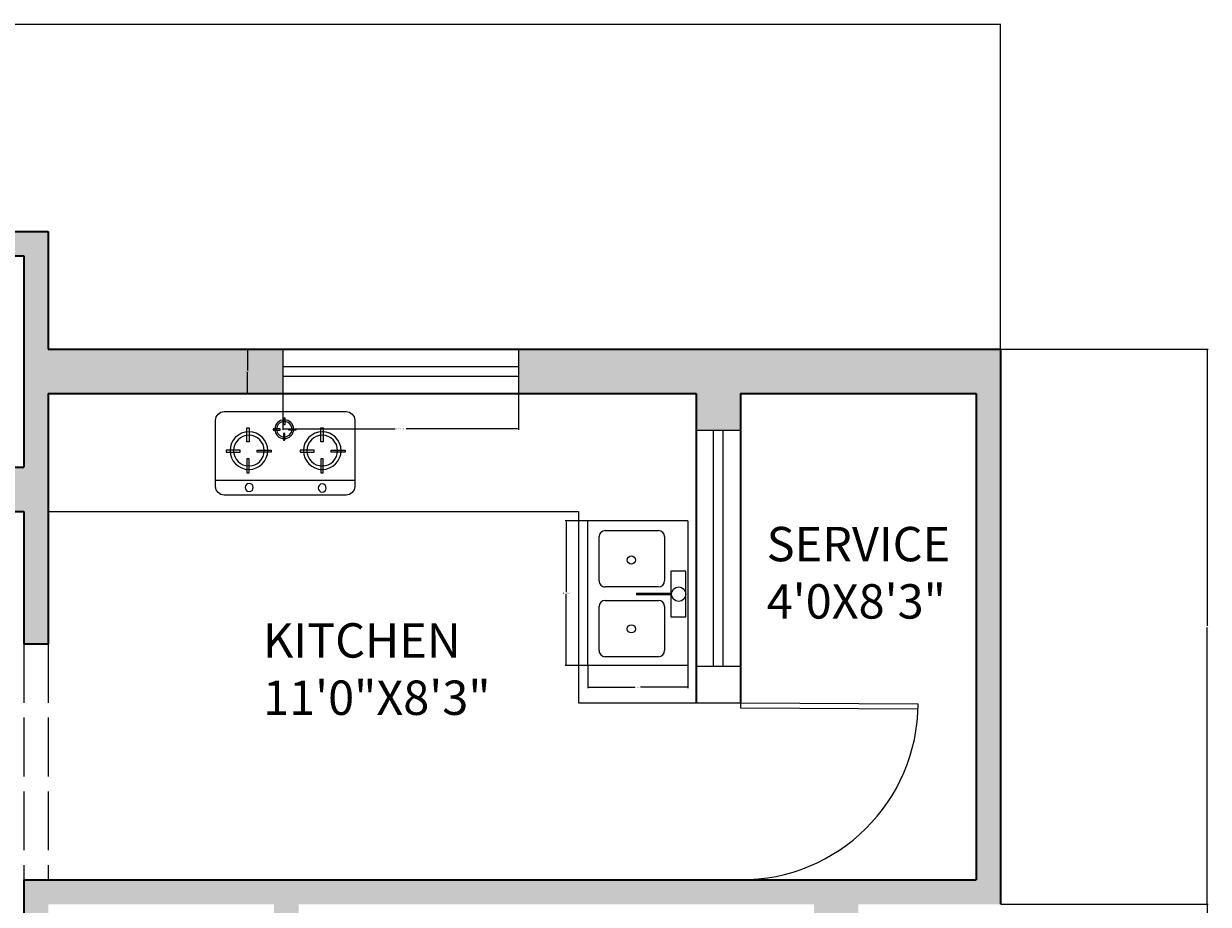
# Model space of a CAD drawing. Units: inches. Extents: x 2540 to 3167, y 3083 to 4007.
# Tile 15 of 15: x 2926 to 3167, y 3828 to 4007. Entities that reach past the tile are written whole.
import ezdxf

# ---------------------------------------------------------------- set-up
doc = ezdxf.new("R2010")
doc.units = ezdxf.units.IN
doc.linetypes.add('ACAD_ISO02W100', pattern=[15, 12, -3])
for name, color, linetype, lineweight in [('A-ANNO-DIMS', 2, 'Continuous', 18), ('A-AREA-IDEN', 7, 'Continuous', 18), ('A-DOOR', 4, 'Continuous', 18), ('A-EQPM', 9, 'Continuous', 18), ('A-FLOR-CASE', 9, 'Continuous', 18), ('A-FLOR-FIXT', 9, 'Continuous', 18), ('A-GLAZ', 4, 'Continuous', 18)]:
    doc.layers.add(name, color=color, linetype=linetype, lineweight=lineweight)
for name, color, linetype, lineweight, true_color in [('A-WALL', 143, 'Continuous', 35, 0x7aafdf), ('A-WALL-OVHD', 143, 'ACAD_ISO02W100', 18, 0x7aafdf), ('A-WALL-PATT', 143, 'Continuous', 13, 0x7aafdf)]:
    doc.layers.add(name, color=color, linetype=linetype, lineweight=lineweight, true_color=true_color)
doc.styles.get("Standard").update_dxf_attribs({"font": 'arial.ttf'})
doc.dimstyles.get("Standard").update_dxf_attribs({"dimtxt": 0.18, "dimasz": 0.18, "dimexe": 0.18, "dimexo": 0.0625, "dimgap": 0.09, "dimtad": 0, "dimtih": 1, "dimtoh": 1, "dimdec": 4, "dimzin": 0, "dimdsep": 46, "dimtxsty": 'Standard', "dimcen": 0.09, "dimadec": 0, "dimazin": 0, "dimtfac": 1, "dimtdec": 4, "dimtofl": 0, "dimtmove": 0, "dimatfit": 3, "dimfxl": 1, "dimtolj": 1, "dimtzin": 0, "dimarcsym": 0})

# ---------------------------------------------------------------- blocks, each defined once
blk = doc.blocks.new('A$C2A3C6842')
for p, q in [((45, 432), (675, 432)), ((0, 45), (0, 387)), ((351.6, 363.3), (351.6, 398.9)), ((351.6, 398.9), (357.3, 398.9)), ((357.3, 398.9), (357.3, 363.3)), ((720, 387), (720, 45)), ((161.8, 346.9), (173.2, 346.9)), ((161.8, 275.6), (161.8, 346.9)), ((173.2, 346.9), (173.2, 275.6)), ((298.4, 341.9), (298.4, 336.2)), ((334, 341.9), (298.4, 341.9)), ((298.4, 336.2), (334, 336.2)), ((334, 336.2), (334, 341.9)), ((357.3, 363.3), (351.6, 363.3)), ((357.3, 318.8), (351.6, 318.8)), ((351.6, 318.8), (351.6, 283.1)), ((357.3, 283.1), (357.3, 318.8)), ((378.5, 336.2), (378.5, 341.9)), ((378.5, 341.9), (414.2, 341.9)), ((414.2, 336.2), (378.5, 336.2)), ((414.2, 341.9), (414.2, 336.2)), ((544.7, 346.9), (556.1, 346.9)), ((544.7, 275.6), (544.7, 346.9)), ((556.1, 346.9), (556.1, 275.6)), ((173.2, 275.6), (161.8, 275.6)), ((351.6, 283.1), (357.3, 283.1)), ((556.1, 275.6), (544.7, 275.6)), ((55.3, 232.9), (55.3, 221.5)), ((126.6, 232.9), (55.3, 232.9)), ((55.3, 221.5), (126.6, 221.5)), ((126.6, 221.5), (126.6, 232.9)), ((173.2, 186.6), (161.8, 186.6)), ((161.8, 186.6), (161.8, 115.3)), ((173.2, 115.3), (173.2, 186.6)), ((215.6, 221.5), (215.6, 232.9)), ((215.6, 232.9), (286.9, 232.9)), ((286.9, 221.5), (215.6, 221.5)), ((286.9, 232.9), (286.9, 221.5)), ((438.2, 232.9), (438.2, 221.5)), ((509.5, 232.9), (438.2, 232.9)), ((438.2, 221.5), (509.5, 221.5)), ((509.5, 221.5), (509.5, 232.9)), ((556.1, 186.6), (544.7, 186.6)), ((544.7, 186.6), (544.7, 115.3)), ((556.1, 115.3), (556.1, 186.6)), ((598.5, 232.9), (669.8, 232.9)), ((598.5, 221.5), (598.5, 232.9)), ((669.8, 221.5), (598.5, 221.5)), ((669.8, 232.9), (669.8, 221.5)), ((1.2, 76.7), (719.9, 76.7)), ((161.8, 115.3), (173.2, 115.3)), ((544.7, 115.3), (556.1, 115.3)), ((675, 0), (45, 0))]:
    blk.add_line(p, q)
at = {"extrusion": (0, -1e-16, -1)}
for centre, major_axis, start_param, end_param in [((45, 387), (31.8, 31.8), 3.926991, 5.497787), ((172.2, 229.8), (-97.3, 0.1), -0.001099, 6.282086), ((551.8, 229.8), (-97.3, 0.1), -0.001099, 6.282086), ((173.7, 39), (-14.8, 14.8), 5.497787, 11.780972)]:
    blk.add_ellipse(centre, major_axis=major_axis, ratio=1, start_param=start_param, end_param=end_param, dxfattribs=at)
at = {"extrusion": (0, 1e-16, -1)}
blk.add_ellipse((675, 387), major_axis=(-31.8, 31.8), ratio=1, start_param=0.785398, end_param=2.356194, dxfattribs=at)
at = {"extrusion": (-1e-16, -1e-16, -1)}
blk.add_ellipse((355.1, 340.4), major_axis=(48.7, 0.1), ratio=1, start_param=3.144125, end_param=9.42731, dxfattribs=at)
at = {"extrusion": (-1e-16, 0, -1)}
for centre, major_axis, start_param, end_param in [((355.1, 340.4), (-39.7, 0), -0.000334, 6.282851), ((45, 45), (-31.8, 31.8), 3.926991, 5.497787)]:
    blk.add_ellipse(centre, major_axis=major_axis, ratio=1, start_param=start_param, end_param=end_param, dxfattribs=at)
at = {"extrusion": (-1e-16, -4e-16, -1)}
for centre in [(172.2, 229.8), (551.8, 229.8)]:
    blk.add_ellipse(centre, major_axis=(-79.3, 0), ratio=1, start_param=-0.0002116186602152, end_param=6.282973688519371, dxfattribs=at)
at = {"extrusion": (2e-16, -2e-16, -1)}
blk.add_ellipse((551.4, 36.4), major_axis=(14.8, 14.8), ratio=1, start_param=3.926991, end_param=10.210176, dxfattribs=at)
at = {"extrusion": (-2e-16, 1e-16, -1)}
blk.add_ellipse((675, 45), major_axis=(31.8, 31.8), ratio=1, start_param=0.785398, end_param=2.356194, dxfattribs=at)
at = {"text_generation_flag": 4, "flags": 9}
for tag in ['XSIZE', 'YSIZE']:
    blk.add_attdef(tag, (361.3, 264.9), '', height=0.45, rotation=180, dxfattribs=at)
blk = doc.blocks.new('A$C3AD04490')
for p, q in [((0, 640.7), (0, 0)), ((0, 640.7), (924.9, 640.7)), ((614, 627.3), (322.5, 627.3)), ((322.5, 627.3), (322.5, 531.5)), ((614, 531.5), (614, 627.3)), ((924.9, 640.7), (924.9, 0)), ((322.5, 531.5), (614, 531.5)), ((462.6, 311.9), (462.6, 537.2)), ((473.8, 536.8), (473.8, 311.9)), ((101.4, 490.5), (383.1, 490.5)), ((547.9, 490.5), (829.6, 490.5)), ((62.3, 110.9), (62.3, 451.4)), ((422.3, 451.4), (422.3, 110.9)), ((508.8, 110.9), (508.8, 451.4)), ((868.8, 451.4), (868.8, 110.9)), ((463.4, 310.9), (474.3, 310.9)), ((383.1, 71.7), (101.4, 71.7)), ((829.6, 71.7), (547.9, 71.7)), ((924.9, 0), (0, 0))]:
    blk.add_line(p, q)
for centre, radius in [((469, 581.2), 45.9), ((250.7, 278.1), 26.4), ((690.5, 278.1), 26.4)]:
    blk.add_circle(centre, radius)
for centre, start, end in [((101.4, 451.4), 90, 180), ((383.1, 451.4), 0, 90), ((547.9, 451.4), 90, 180), ((829.6, 451.4), 0, 90), ((101.4, 110.9), 180, 270), ((383.1, 110.9), 270, 0), ((547.9, 110.9), 180, 270), ((829.6, 110.9), 270, 0)]:
    blk.add_arc(centre, 39.1, start, end)
blk = doc.blocks.new('WIN-48IN')
for p, q in [((0, 48), (9, 48)), ((3.5, 0), (3.5, 48)), ((5.5, 0), (5.5, 48)), ((0, 0), (9, 0))]:
    blk.add_line(p, q)
blk = doc.blocks.new('*D25')
at = {"layer": 'A-ANNO-DIMS', "color": 0, "lineweight": -2, "transparency": 16777216}
for p, q in [((2978.28, 3931.65), (2978.28, 3924.33)), ((3026.28, 3931.65), (3026.28, 3924.33)), ((2978.46, 3924.51), (3001.16, 3924.51)), ((3026.1, 3924.51), (3003.4, 3924.51))]:
    blk.add_line(p, q, dxfattribs=at)
at = {"layer": 'A-ANNO-DIMS', "color": 0, "transparency": 16777216}
for points in [[(2978.46, 3924.54), (2978.46, 3924.48), (2978.28, 3924.51)], [(3026.1, 3924.54), (3026.1, 3924.48), (3026.28, 3924.51)]]:
    blk.add_solid(points, dxfattribs=at)
at = {"layer": 'Defpoints', "color": 0, "transparency": 16777216}
for p in [(2978.28, 3931.71), (3026.28, 3931.71), (3026.28, 3924.51)]:
    blk.add_point(p, dxfattribs=at)
at = {"layer": 'A-ANNO-DIMS', "color": 0, "transparency": 16777216, "insert": (3002.28, 3924.51), "char_height": 0.18, "attachment_point": 5}
blk.add_mtext('\\A1;WINDOW 48 TYP.', dxfattribs=at)
blk = doc.blocks.new('*D26')
at = {"layer": 'A-ANNO-DIMS', "color": 0, "lineweight": -2, "transparency": 16777216}
for p, q in [((2978.22, 3940.71), (2970.9, 3940.71)), ((2971.08, 3940.53), (2971.08, 3936.4)), ((2971.08, 3931.89), (2971.08, 3936.03)), ((2978.22, 3931.71), (2970.9, 3931.71))]:
    blk.add_line(p, q, dxfattribs=at)
at = {"layer": 'A-ANNO-DIMS', "color": 0, "transparency": 16777216}
for points in [[(2971.05, 3940.53), (2971.11, 3940.53), (2971.08, 3940.71)], [(2971.05, 3931.89), (2971.11, 3931.89), (2971.08, 3931.71)]]:
    blk.add_solid(points, dxfattribs=at)
at = {"layer": 'Defpoints', "color": 0, "transparency": 16777216}
for p in [(2978.28, 3940.71), (2971.08, 3931.71), (2978.28, 3931.71)]:
    blk.add_point(p, dxfattribs=at)
at = {"layer": 'A-ANNO-DIMS', "color": 0, "transparency": 16777216, "insert": (2971.08, 3936.21), "char_height": 0.18, "attachment_point": 5}
blk.add_mtext('\\A1;9 TYP.', dxfattribs=at)
blk = doc.blocks.new('*D35')
at = {"layer": 'A-ANNO-DIMS', "color": 0, "lineweight": -2, "transparency": 16777216}
for p, q in [((3040.35, 3905.79), (3035.82, 3905.79)), ((3036, 3905.61), (3036, 3891.25)), ((3036, 3876.52), (3036, 3890.88)), ((3040.35, 3876.34), (3035.82, 3876.34))]:
    blk.add_line(p, q, dxfattribs=at)
at = {"layer": 'A-ANNO-DIMS', "color": 0, "transparency": 16777216}
for points in [[(3035.97, 3905.61), (3036.03, 3905.61), (3036, 3905.79)], [(3035.97, 3876.52), (3036.03, 3876.52), (3036, 3876.34)]]:
    blk.add_solid(points, dxfattribs=at)
at = {"layer": 'Defpoints', "color": 0, "transparency": 16777216}
for p in [(3040.42, 3905.79), (3036, 3876.34), (3040.42, 3876.34)]:
    blk.add_point(p, dxfattribs=at)
at = {"layer": 'A-ANNO-DIMS', "color": 0, "transparency": 16777216, "insert": (3036, 3891.06), "char_height": 0.18, "attachment_point": 5}
blk.add_mtext('\\A1;SINK 29 TYP.', dxfattribs=at)
blk = doc.blocks.new('*D36')
at = {"layer": 'A-ANNO-DIMS', "color": 0, "lineweight": -2, "transparency": 16777216}
for p, q in [((3040.42, 3876.27), (3040.42, 3871.74)), ((3060.82, 3876.27), (3060.82, 3871.74)), ((3040.6, 3871.92), (3050.09, 3871.92)), ((3060.64, 3871.92), (3051.15, 3871.92))]:
    blk.add_line(p, q, dxfattribs=at)
at = {"layer": 'A-ANNO-DIMS', "color": 0, "transparency": 16777216}
for points in [[(3040.6, 3871.95), (3040.6, 3871.89), (3040.42, 3871.92)], [(3060.64, 3871.95), (3060.64, 3871.89), (3060.82, 3871.92)]]:
    blk.add_solid(points, dxfattribs=at)
at = {"layer": 'Defpoints', "color": 0, "transparency": 16777216}
for p in [(3040.42, 3876.34), (3060.82, 3876.34), (3060.82, 3871.92)]:
    blk.add_point(p, dxfattribs=at)
at = {"layer": 'A-ANNO-DIMS', "color": 0, "transparency": 16777216, "insert": (3050.62, 3871.92), "char_height": 0.18, "attachment_point": 5}
blk.add_mtext('\\A1;20 TYP.', dxfattribs=at)
blk = doc.blocks.new('*D43')
at = {"layer": 'A-ANNO-DIMS', "color": 0, "lineweight": -2, "transparency": 16777216}
for p, q in [((2582.51, 3940.78), (2582.51, 4006.99)), ((2582.69, 4006.81), (2853.22, 4006.81)), ((3124.33, 4006.81), (2853.8, 4006.81)), ((3124.51, 3940.78), (3124.51, 4006.99))]:
    blk.add_line(p, q, dxfattribs=at)
at = {"layer": 'A-ANNO-DIMS', "color": 0, "transparency": 16777216}
for points in [[(2582.69, 4006.84), (2582.69, 4006.78), (2582.51, 4006.81)], [(3124.33, 4006.84), (3124.33, 4006.78), (3124.51, 4006.81)]]:
    blk.add_solid(points, dxfattribs=at)
at = {"layer": 'Defpoints', "color": 0, "transparency": 16777216}
for p in [(3124.51, 4006.81), (2582.51, 3940.71), (3124.51, 3940.71)]:
    blk.add_point(p, dxfattribs=at)
at = {"layer": 'A-ANNO-DIMS', "color": 0, "transparency": 16777216, "insert": (2853.51, 4006.81), "char_height": 0.18, "attachment_point": 5}
blk.add_mtext('\\A1;542', dxfattribs=at)
blk = doc.blocks.new('*D48')
at = {"layer": 'A-ANNO-DIMS', "color": 0, "lineweight": -2, "transparency": 16777216}
for p, q in [((3124.57, 3940.71), (3166.79, 3940.71)), ((3166.61, 3940.53), (3166.61, 3884.4)), ((3166.61, 3827.89), (3166.61, 3884.03)), ((3124.57, 3827.71), (3166.79, 3827.71))]:
    blk.add_line(p, q, dxfattribs=at)
at = {"layer": 'A-ANNO-DIMS', "color": 0, "transparency": 16777216}
for points in [[(3166.58, 3940.53), (3166.64, 3940.53), (3166.61, 3940.71)], [(3166.58, 3827.89), (3166.64, 3827.89), (3166.61, 3827.71)]]:
    blk.add_solid(points, dxfattribs=at)
at = {"layer": 'Defpoints', "color": 0, "transparency": 16777216}
for p in [(3124.51, 3940.71), (3124.51, 3827.71), (3166.61, 3827.71)]:
    blk.add_point(p, dxfattribs=at)
at = {"layer": 'A-ANNO-DIMS', "color": 0, "transparency": 16777216, "insert": (3166.61, 3884.21), "char_height": 0.18, "attachment_point": 5}
blk.add_mtext('\\A1;113', dxfattribs=at)
blk = doc.blocks.new('*D49')
at = {"layer": 'A-ANNO-DIMS', "color": 0, "lineweight": -2, "transparency": 16777216}
for p, q in [((3124.57, 3827.71), (3166.79, 3827.71)), ((3166.61, 3827.53), (3166.61, 3727.9)), ((3166.61, 3627.89), (3166.61, 3727.53)), ((3124.57, 3627.71), (3166.79, 3627.71))]:
    blk.add_line(p, q, dxfattribs=at)
at = {"layer": 'A-ANNO-DIMS', "color": 0, "transparency": 16777216}
for points in [[(3166.58, 3827.53), (3166.64, 3827.53), (3166.61, 3827.71)], [(3166.58, 3627.89), (3166.64, 3627.89), (3166.61, 3627.71)]]:
    blk.add_solid(points, dxfattribs=at)
at = {"layer": 'Defpoints', "color": 0, "transparency": 16777216}
for p in [(3124.51, 3827.71), (3124.51, 3627.71), (3166.61, 3627.71)]:
    blk.add_point(p, dxfattribs=at)
at = {"layer": 'A-ANNO-DIMS', "color": 0, "transparency": 16777216, "insert": (3166.61, 3727.71), "char_height": 0.18, "attachment_point": 5}
blk.add_mtext('\\A1;200', dxfattribs=at)

msp = doc.modelspace()

# ---------------------------------------------------------------- hatches: boundary and pattern name
at = {"layer": 'A-WALL-PATT'}
h = msp.add_hatch(color=256, dxfattribs=at)
h.dxf.hatch_style = 1
h.paths.add_polyline_path([(2644.77, 3940.71), (2582.51, 3940.71), (2582.51, 3886.71), (2612.51, 3886.71), (2612.51, 3871.71), (2621.51, 3871.71), (2621.51, 3895.71), (2591.51, 3895.71), (2591.51, 3931.71), (2621.51, 3931.71), (2644.77, 3931.71)])
h.paths.add_polyline_path([(2746.51, 3940.71), (2716.77, 3940.71), (2716.77, 3931.71), (2741.51, 3931.71), (2741.51, 3839.71), (2748.51, 3839.71), (2748.51, 3844.71), (2746.51, 3844.71), (2746.51, 3931.71)])
h.paths.add_polyline_path([(2805.51, 3959.71), (2925.51, 3959.71), (2925.51, 3916.71), (2913.51, 3916.71), (2913.51, 3907.71), (2925.51, 3907.71), (2925.51, 3880.71), (2930.51, 3880.71), (2930.51, 3931.71), (2978.28, 3931.71), (2978.28, 3940.71), (2930.51, 3940.71), (2930.51, 3964.71), (2800.51, 3964.71), (2800.51, 3940.71), (2776.51, 3940.71), (2776.51, 3964.71), (2771.51, 3964.71), (2771.51, 3940.71), (2771.51, 3931.71), (2800.51, 3931.71), (2800.51, 3839.71), (2805.51, 3839.71), (2805.51, 3907.71), (2817.48, 3907.71), (2817.48, 3916.71), (2805.51, 3916.71)])
h.paths.add_polyline_path([(3124.51, 3940.71), (3026.28, 3940.71), (3026.28, 3931.71), (3062.51, 3931.71), (3062.51, 3924.21), (3071.51, 3924.21), (3071.51, 3931.71), (3119.51, 3931.71), (3119.51, 3832.71), (2925.51, 3832.71), (2925.51, 3815.71), (2930.51, 3815.71), (2930.51, 3827.71), (2976.51, 3827.71), (2976.51, 3773.71), (2970.51, 3773.71), (2970.51, 3768.71), (2985.51, 3768.71), (2985.51, 3773.71), (2981.51, 3773.71), (2981.51, 3827.71), (3086.51, 3827.71), (3086.51, 3812.71), (3095.51, 3812.71), (3095.51, 3827.71), (3124.51, 3827.71)])

# ---------------------------------------------------------------- linework, layer by layer
at = {"layer": 'A-DOOR'}
for p, q in [((3071.51, 3868.71), (3107.71, 3868.51)), ((3071.51, 3868.71), (3071.51, 3867.71)), ((3071.51, 3867.71), (3107.69, 3867.51))]:
    msp.add_line(p, q, dxfattribs=at)
msp.add_arc((3071.71, 3868.71), 36, 269.6785, 359.6785, dxfattribs=at)
at = {"layer": 'A-FLOR-CASE'}
for p, q in [((2930.51, 3907.71), (3038.51, 3907.71)), ((3038.51, 3907.71), (3038.51, 3868.71)), ((3038.51, 3868.71), (3071.51, 3868.71))]:
    msp.add_line(p, q, dxfattribs=at)
at = {"layer": 'A-WALL'}
for p, q in [((2800.51, 3964.71), (2930.51, 3964.71)), ((2930.51, 3964.71), (2930.51, 3940.71)), ((2805.51, 3959.71), (2925.51, 3959.71)), ((2925.51, 3959.71), (2925.51, 3916.71)), ((2930.51, 3940.71), (3124.51, 3940.71)), ((3124.51, 3940.71), (3124.51, 3827.71)), ((2930.51, 3931.71), (3062.51, 3931.71)), ((2930.51, 3931.71), (2930.51, 3880.71)), ((3062.51, 3931.71), (3062.51, 3868.71)), ((3071.51, 3931.71), (3071.51, 3868.71)), ((3071.51, 3931.71), (3119.51, 3931.71)), ((3119.51, 3931.71), (3119.51, 3832.71)), ((2913.51, 3916.71), (2925.51, 3916.71)), ((2913.51, 3907.71), (2925.51, 3907.71)), ((2925.51, 3907.71), (2925.51, 3880.71)), ((2925.51, 3880.71), (2930.51, 3880.71)), ((2925.51, 3832.71), (3119.51, 3832.71)), ((2925.51, 3832.71), (2925.51, 3815.71))]:
    msp.add_line(p, q, dxfattribs=at)
at = {"layer": 'A-WALL-OVHD'}
for p, q in [((2925.51, 3880.71), (2925.51, 3832.71)), ((2930.51, 3880.71), (2930.51, 3832.71))]:
    msp.add_line(p, q, dxfattribs=at)

# ---------------------------------------------------------------- block references
at = {"layer": 'A-EQPM', "xscale": 0.0393700787401575, "yscale": 0.0393700787401575, "zscale": 0.0393700787401575}
msp.add_blockref('A$C2A3C6842', (2964.61, 3911.03), dxfattribs=at)
at = {"layer": 'A-FLOR-FIXT', "xscale": 0.0318479740928733, "yscale": 0.0318479740928733, "zscale": 0.0318479740928733, "rotation": 270}
msp.add_blockref('A$C3AD04490', (3040.42, 3905.79), dxfattribs=at)
at = {"layer": 'A-GLAZ', "rotation": 269.9999999999988}
msp.add_blockref('WIN-48IN', (2978.28, 3940.71), dxfattribs=at)
at = {"layer": 'A-GLAZ'}
msp.add_blockref('WIN-48IN', (3062.51, 3876.21), dxfattribs=at)

# ---------------------------------------------------------------- texts
at = {"layer": 'A-AREA-IDEN', "char_height": 7, "attachment_point": 1}
for s, width, insert in [('SERVICE\\P4\'0X8\'3"', 37.9387, (3076.85, 3904.55)), ('KITCHEN\\P11\'0"X8\'3"', 74.3296, (2974.27, 3884.94))]:
    msp.add_mtext_dynamic_manual_height_columns(s, width=width, gutter_width=12.5, heights=[0], dxfattribs=dict(at, insert=insert))

# ---------------------------------------------------------------- dimensions: what is measured, and where the dimension line sits
at = {"layer": 'A-ANNO-DIMS'}
dim = msp.add_linear_dim(base=(3124.51, 4006.81), p1=(2582.51, 3940.71), p2=(3124.51, 3940.71), dimstyle='Standard', override={"dimdec": 0, "dimlfac": 1, "dimrnd": 0, "dimzin": 0, "dimdsep": 46, "dimlunit": 2}, dxfattribs=at)
dim.commit()
dim.dimension.update_dxf_attribs({"geometry": '*D43', "text_midpoint": (2853.51, 4006.81)})
for base, p1, p2, text, picture, middle in [((2971.08, 3931.71), (2978.28, 3940.71), (2978.28, 3931.71), '<> TYP.', '*D26', (2971.08, 3936.21)), ((3036, 3876.34), (3040.42, 3905.79), (3040.42, 3876.34), 'SINK <> TYP.', '*D35', (3036, 3891.06))]:
    dim = msp.add_linear_dim(base=base, p1=p1, p2=p2, angle=270, text=text, dimstyle='Standard', override={"dimdec": 0, "dimlfac": 1, "dimrnd": 0, "dimzin": 0, "dimdsep": 46, "dimlunit": 2}, dxfattribs=at)
    dim.commit()
    dim.dimension.update_dxf_attribs({"geometry": picture, "text_midpoint": middle})
for base, p1, p2, picture, middle in [((3166.61, 3827.71), (3124.51, 3940.71), (3124.51, 3827.71), '*D48', (3166.61, 3884.21)), ((3166.61, 3627.71), (3124.51, 3827.71), (3124.51, 3627.71), '*D49', (3166.61, 3727.71))]:
    dim = msp.add_linear_dim(base=base, p1=p1, p2=p2, angle=90, dimstyle='Standard', override={"dimdec": 0, "dimlfac": 1, "dimrnd": 0, "dimzin": 0, "dimdsep": 46, "dimlunit": 2}, dxfattribs=at)
    dim.commit()
    dim.dimension.update_dxf_attribs({"geometry": picture, "text_midpoint": middle})
for base, p1, p2, text, picture, middle in [((3026.28, 3924.51), (2978.28, 3931.71), (3026.28, 3931.71), 'WINDOW <> TYP.', '*D25', (3002.28, 3924.51)), ((3060.82, 3871.92), (3040.42, 3876.34), (3060.82, 3876.34), '<> TYP.', '*D36', (3050.62, 3871.92))]:
    dim = msp.add_linear_dim(base=base, p1=p1, p2=p2, text=text, dimstyle='Standard', override={"dimdec": 0, "dimlfac": 1, "dimrnd": 0, "dimzin": 0, "dimdsep": 46, "dimlunit": 2}, dxfattribs=at)
    dim.commit()
    dim.dimension.update_dxf_attribs({"geometry": picture, "text_midpoint": middle})

doc.saveas('drawing.dxf')
